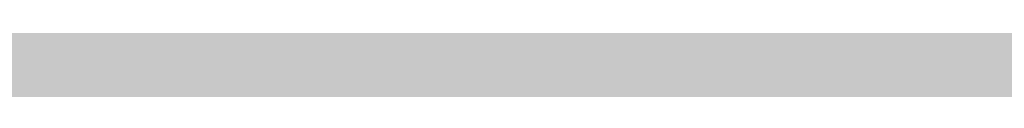
# Model space of a CAD drawing. Units: feet. Extents: x 3168 to 4724, y 827 to 1477.
# Tile 133 of 256: x 3300.8583 to 3301.1298, y 1099.0007 to 1099.0148. Entities that reach past the tile are written whole.
import ezdxf

# ---------------------------------------------------------------- set-up
doc = ezdxf.new("R2010")
doc.units = ezdxf.units.FT
doc.layers.add('A-ELEV', color=7, linetype='Continuous', lineweight=35)
doc.layers.add('A-ELEV-PATT', color=8, linetype='Continuous', lineweight=13)

msp = doc.modelspace()

# ---------------------------------------------------------------- hatches: boundary and pattern name
at = {"layer": 'A-ELEV-PATT'}
h = msp.add_hatch(color=256, dxfattribs=at)
h.dxf.hatch_style = 1
edge = h.paths.add_edge_path()
edge.add_ellipse((3552.90576, 979.22014), major_axis=(36.74492, 0), ratio=0.48484848, start_angle=0, end_angle=360)
edge = h.paths.add_edge_path()
edge.add_ellipse((3559.89164, 929.25228), major_axis=(36.74492, 0), ratio=0.48484848, start_angle=0, end_angle=360)
edge = h.paths.add_edge_path()
edge.add_line((3299.31681, 1198.60608), (3479.91671, 1198.60608))
edge.add_line((3479.91671, 1198.60608), (3479.91671, 1209.86857))
edge.add_spline(control_points=[(3479.91671, 1209.86857), (3464.30116, 1209.86857), (3448.6856, 1209.86857), (3410.94914, 1209.86857), (3388.82823, 1209.86857), (3355.64688, 1209.86857), (3344.58642, 1209.86857), (3327.99574, 1209.86857), (3322.46552, 1209.86857), (3314.17018, 1209.86857), (3311.40507, 1209.86857), (3307.2574, 1209.86857), (3305.87484, 1209.86857), (3303.801, 1209.86857), (3303.10973, 1209.86857), (3302.07281, 1209.86857), (3301.72717, 1209.86857), (3301.20871, 1209.86857), (3301.03589, 1209.86857), (3300.77666, 1209.86857), (3300.69025, 1209.86857), (3300.56064, 1209.86857), (3300.51743, 1209.86857), (3300.45263, 1209.86857), (3300.43102, 1209.86857), (3300.39862, 1209.86857), (3300.38782, 1209.86857), (3300.36622, 1209.86857), (3300.34568, 1209.86857), (3300.34555, 1209.86857), (3300.3455, 1209.86857), (3300.3433, 1209.86857), (3300.34115, 1209.86857), (3300.33791, 1209.86857), (3300.33683, 1209.86857), (3300.33394, 1209.86857), (3300.33213, 1209.86857), (3300.32552, 1209.86858), (3300.32071, 1209.86858), (3300.31092, 1209.86859), (3300.30595, 1209.8686), (3300.29051, 1209.86862), (3300.28005, 1209.86865), (3300.23243, 1209.86878), (3300.1953, 1209.86895), (3299.95107, 1209.87061), (3299.74482, 1209.87433), (3299.43683, 1209.88326), (3299.33439, 1209.88679), (3299.18108, 1209.89292), (3299.13003, 1209.8951), (3298.65222, 1209.9168), (3298.22946, 1209.94572), (3297.60163, 1210.00237), (3297.3934, 1210.02346), (3297.08265, 1210.05831), (3296.97933, 1210.07046), (3296.29295, 1210.15486), (3295.71815, 1210.24336), (3294.86872, 1210.39885), (3294.5877, 1210.45448), (3294.16934, 1210.54335), (3294.03042, 1210.57388), (3291.70715, 1211.1012), (3289.65359, 1211.81344), (3285.77626, 1213.56399), (3283.95141, 1214.60348), (3280.51216, 1216.98008), (3278.89724, 1218.31759), (3276.37991, 1220.82949), (3275.41604, 1221.91774), (3274.03934, 1223.7077), (3273.58104, 1224.34953), (3273.14323, 1225.01632)], knot_values=[39.119033, 39.119033, 39.119033, 39.119033, 39.286353, 39.286353, 39.523379, 39.523379, 39.641892, 39.641892, 39.701148, 39.701148, 39.730777, 39.730777, 39.745591, 39.745591, 39.752998, 39.752998, 39.756701, 39.756701, 39.758553, 39.758553, 39.759479, 39.759479, 39.759942, 39.759942, 39.760173, 39.760173, 39.760289, 39.760289, 39.760405, 39.760405, 39.760463, 39.760463, 39.763389, 39.763389, 39.764851, 39.764851, 39.767304, 39.767304, 39.773825, 39.773825, 39.78057, 39.78057, 39.79477, 39.79477, 39.845194, 39.845194, 40.126715, 40.126715, 40.267476, 40.267476, 40.337856, 40.337856, 40.927023, 40.927023, 41.221606, 41.221606, 41.368898, 41.368898, 42.202622, 42.202622, 42.619485, 42.619485, 42.827916, 42.827916, 46.118323, 46.118323, 49.408731, 49.408731, 52.699139, 52.699139, 54.927489, 54.927489, 56.104228, 56.104228, 56.104228, 56.104228], weights=[1, 1, 1, 1, 1, 1, 1, 1, 1, 1, 1, 1, 1, 1, 1, 1, 1, 1, 1, 1, 1, 1, 1, 1, 1, 1, 1, 1, 1, 1, 1, 1, 1, 1, 1, 1, 1, 1, 1, 1, 1, 1, 1, 1, 1, 1, 1, 1, 1, 1, 1, 1, 1, 1, 1, 1, 1, 1, 1, 1, 1, 1, 1, 1, 1, 1, 1, 1, 1, 1, 1, 1, 1, 1], degree=3, periodic=0)
edge.add_line((3273.14323, 1225.01632), (3273.14323, 1099.01632))
edge.add_line((3273.14323, 1099.01632), (3299.31681, 1099.01632))
edge.add_line((3299.31681, 1099.01632), (3299.31681, 1198.60608))
edge = h.paths.add_edge_path()
edge.add_line((3304.75844, 1324.15806), (3479.91671, 1324.15806))
edge.add_line((3479.91671, 1324.15806), (3479.91671, 1335.71462))
edge.add_line((3479.91671, 1335.71462), (3269.16163, 1335.71462))
edge.add_spline(control_points=[(3269.16163, 1335.71462), (3264.02423, 1335.71462), (3258.36412, 1328.95819), (3259.26431, 1323.90027)], knot_values=[0, 0, 0, 0, 15.412191, 15.412191, 15.412191, 15.412191], degree=3, periodic=0)
edge.add_line((3259.26431, 1323.90027), (3265.51685, 1288.76913))
edge.add_line((3265.51685, 1288.76913), (3275.2651, 1261.54563))
edge.add_line((3275.2651, 1261.54563), (3304.75844, 1261.54563))
edge.add_line((3304.75844, 1261.54563), (3304.75844, 1324.15806))
h = msp.add_hatch(color=256, dxfattribs=at)
h.dxf.hatch_style = 1
h.paths.add_polyline_path([(3384.52525, 1099.01632), (3335.02917, 1099.01632), (3299.31681, 1099.01632), (3273.14323, 1099.01632), (3217.56536, 1099.01632), (3168.06928, 827.11626), (3335.02917, 827.11626)])

# ---------------------------------------------------------------- linework, layer by layer
at = {"layer": 'A-ELEV'}
msp.add_open_spline([(3808.5202, 1099.01632), (3808.5202, 1141.41324), (3808.5202, 1183.81015), (3808.5202, 1226.63532), (3808.5202, 1227.06358), (3808.5202, 1227.49183), (3811.49187, 1248.99467), (3814.46354, 1270.49752), (3817.46523, 1292.21756), (3817.49525, 1292.43476), (3817.52526, 1292.65196), (3817.5728, 1310.10675), (3817.62034, 1327.56153), (3817.66788, 1345.01632), (3817.66788, 1345.45796), (3817.66788, 1345.89961), (3817.66788, 1346.45605), (3817.66788, 1346.57084), (3817.66788, 1346.75289), (3817.66788, 1346.82014), (3817.66788, 1346.93487), (3817.66788, 1346.98234), (3817.66788, 1347.03859), (3817.66788, 1347.04736), (3817.66788, 1347.07366), (3817.66788, 1347.0593), (3817.66788, 1347.06155), (3817.66788, 1347.06267), (3817.66788, 1347.06603), (3817.66787, 1347.06827), (3817.66787, 1347.075), (3817.66787, 1347.07949), (3817.66785, 1347.09294), (3817.66783, 1347.1019), (3817.66777, 1347.12879), (3817.6677, 1347.1467), (3817.66743, 1347.20042), (3817.66716, 1347.23619), (3817.6661, 1347.34338), (3817.66504, 1347.41469), (3817.66081, 1347.62809), (3817.65661, 1347.76971), (3817.63997, 1348.19249), (3817.62351, 1348.47159), (3817.55909, 1349.30007), (3817.49612, 1349.84059), (3817.25543, 1351.42416), (3817.02632, 1352.42879), (3816.30687, 1354.88891), (3815.74375, 1356.26873), (3814.46396, 1358.81921), (3813.74641, 1359.99097), (3812.19584, 1362.17234), (3811.36225, 1363.18212), (3809.58884, 1365.06901), (3808.64882, 1365.94611), (3806.65426, 1367.57962), (3805.5997, 1368.33615), (3803.35289, 1369.72233), (3802.16054, 1370.35239), (3799.60081, 1371.45359), (3798.23269, 1371.92548), (3795.28008, 1372.63462), (3793.69315, 1372.87207), (3791.86944, 1372.92648), (3791.74086, 1372.92922), (3791.35337, 1372.9341), (3791.09271, 1372.9329), (3790.30412, 1372.91507), (3789.76954, 1372.88419), (3789.20919, 1372.83024), (3789.19062, 1372.82842), (3789.13489, 1372.82291), (3789.0977, 1372.81914), (3789.04844, 1372.81401), (3789.0364, 1372.81274), (3789.00026, 1372.80892), (3788.97615, 1372.80633), (3788.9494, 1372.8034), (3788.94679, 1372.80312), (3788.94257, 1372.80266), (3788.94097, 1372.80248), (3788.93857, 1372.80222), (3788.93778, 1372.80213), (3788.93539, 1372.80187), (3788.86753, 1372.7944), (3788.75687, 1372.78223), (3788.70153, 1372.77614), (3788.53553, 1372.75788), (3788.42486, 1372.74571), (3788.09286, 1372.70918), (3787.87152, 1372.68484), (3787.20751, 1372.61179), (3786.76483, 1372.5631), (3785.43681, 1372.41701), (3784.55147, 1372.31962), (3781.89542, 1372.02744), (3780.12473, 1371.83266), (3774.81265, 1371.24831), (3771.27126, 1370.85874), (3760.64709, 1369.69004), (3753.56431, 1368.9109), (3732.31597, 1366.5735), (3718.15042, 1365.01523), (3694.00676, 1362.35933), (3684.02866, 1361.26169), (3674.05056, 1360.16406), (3664.60066, 1360.16406), (3655.15077, 1360.16406), (3626.80108, 1360.16406), (3607.90129, 1360.16406), (3551.20192, 1360.16406), (3513.40234, 1360.16406), (3467.72518, 1360.16406), (3459.8476, 1360.16406), (3436.21487, 1360.16406), (3420.45972, 1360.16406), (3373.19425, 1360.16406), (3341.68395, 1360.16406), (3302.84816, 1360.16406), (3295.52269, 1360.16406), (3286.03829, 1360.16406), (3283.87937, 1360.16406), (3277.40261, 1360.16406), (3273.08477, 1360.16406), (3267.73285, 1360.16406), (3266.69877, 1360.16406), (3263.59652, 1360.16406), (3261.52835, 1360.16406), (3259.23694, 1360.16406), (3259.0137, 1360.16406), (3258.34396, 1360.16406), (3257.89747, 1360.16406), (3257.431, 1360.16406), (3257.41102, 1360.16406), (3257.37057, 1360.16406), (3257.37547, 1360.16406), (3257.3746, 1360.16406), (3257.37394, 1360.16406), (3257.37196, 1360.16406), (3257.37064, 1360.16406), (3257.36667, 1360.16406), (3257.36403, 1360.16406), (3257.35611, 1360.16405), (3257.35083, 1360.16405), (3257.33499, 1360.16402), (3257.32443, 1360.164), (3257.29277, 1360.1639), (3257.27168, 1360.1638), (3257.20844, 1360.1634), (3257.16634, 1360.163), (3257.04021, 1360.16139), (3256.95635, 1360.15978), (3256.7055, 1360.15339), (3256.53924, 1360.14704), (3256.04357, 1360.12192), (3255.7173, 1360.0971), (3254.75245, 1360.00048), (3254.12797, 1359.90651), (3252.18007, 1359.52533), (3250.94157, 1359.14399), (3248.67018, 1358.24329), (3247.63574, 1357.72383), (3245.73263, 1356.60347), (3244.86339, 1356.00206), (3243.25311, 1354.74287), (3242.51197, 1354.08473), (3240.75105, 1352.34478), (3239.80096, 1351.22957), (3238.08777, 1348.87244), (3237.32469, 1347.63036), (3235.98251, 1344.97163), (3235.40221, 1343.55491), (3234.59108, 1340.81546), (3234.31088, 1339.54355), (3233.97649, 1336.80256), (3233.92211, 1335.33088), (3234.14892, 1332.59127), (3234.34953, 1331.3672), (3234.71989, 1329.99937), (3234.75242, 1329.88336), (3234.85362, 1329.5348), (3234.92589, 1329.30168), (3235.02484, 1329.00255), (3235.04692, 1328.93693), (3235.07764, 1328.84724), (3235.08592, 1328.8232), (3235.11094, 1328.75106), (3235.12783, 1328.70296), (3235.14799, 1328.64624), (3235.15106, 1328.63763), (3235.1561, 1328.62353), (3235.15806, 1328.61803), (3235.16021, 1328.61203), (3235.16561, 1328.59694), (3235.1801, 1328.55649), (3235.19026, 1328.5281), (3235.22076, 1328.44295), (3235.24108, 1328.38618), (3235.30207, 1328.21587), (3235.34273, 1328.10232), (3235.4647, 1327.7617), (3235.54601, 1327.53462), (3235.78995, 1326.85338), (3235.95258, 1326.39922), (3236.44046, 1325.03674), (3236.76571, 1324.12841), (3237.74148, 1321.40345), (3238.39198, 1319.5868), (3240.34351, 1314.13687), (3241.64452, 1310.50358), (3245.54757, 1299.60371), (3248.14961, 1292.33713), (3255.95571, 1270.53739), (3261.15977, 1256.00423), (3267.38762, 1238.612), (3268.4114, 1235.75294), (3269.51038, 1232.68386), (3269.58558, 1232.47385), (3269.70661, 1232.13585), (3269.75244, 1232.00786), (3269.82733, 1231.79873), (3269.85638, 1231.7176), (3269.90632, 1231.57812), (3269.92721, 1231.51978), (3269.97247, 1231.39341), (3269.99683, 1231.32537), (3270.0265, 1231.24251), (3270.03181, 1231.22768), (3270.04028, 1231.20402), (3270.03922, 1231.20698), (3270.03936, 1231.2066), (3270.03943, 1231.20641), (3270.03963, 1231.20585), (3270.03977, 1231.20547), (3270.04017, 1231.20433), (3270.04044, 1231.20358), (3270.04125, 1231.20131), (3270.0418, 1231.1998), (3270.04342, 1231.19527), (3270.0445, 1231.19225), (3270.04776, 1231.18318), (3270.04993, 1231.17714), (3270.05644, 1231.15903), (3270.06079, 1231.14696), (3270.07387, 1231.11076), (3270.08261, 1231.08666), (3270.10894, 1231.01441), (3270.1266, 1230.96635), (3270.17993, 1230.82246), (3270.21595, 1230.72692), (3270.32532, 1230.44151), (3270.40003, 1230.25281), (3270.62925, 1229.69144), (3270.78888, 1229.3235), (3271.28649, 1228.23832), (3271.6431, 1227.53975), (3272.77586, 1225.51528), (3273.61417, 1224.2605), (3275.41604, 1221.91774), (3276.37991, 1220.82949), (3278.89724, 1218.31759), (3280.51216, 1216.98008), (3283.95141, 1214.60348), (3285.77626, 1213.56399), (3289.65359, 1211.81344), (3291.70715, 1211.1012), (3294.03042, 1210.57388), (3294.16934, 1210.54335), (3294.5877, 1210.45448), (3294.86872, 1210.39885), (3295.71815, 1210.24336), (3296.29295, 1210.15486), (3296.97933, 1210.07046), (3297.08265, 1210.05831), (3297.3934, 1210.02346), (3297.60163, 1210.00237), (3298.22946, 1209.94572), (3298.65222, 1209.9168), (3299.13003, 1209.8951), (3299.18108, 1209.89292), (3299.33439, 1209.88679), (3299.43683, 1209.88326), (3299.74482, 1209.87433), (3299.95107, 1209.87061), (3300.1953, 1209.86895), (3300.23243, 1209.86878), (3300.28005, 1209.86865), (3300.29051, 1209.86862), (3300.30595, 1209.8686), (3300.31092, 1209.86859), (3300.32071, 1209.86858), (3300.32552, 1209.86858), (3300.33213, 1209.86857), (3300.33394, 1209.86857), (3300.33683, 1209.86857), (3300.33791, 1209.86857), (3300.34115, 1209.86857), (3300.3433, 1209.86857), (3300.3455, 1209.86857), (3300.34555, 1209.86857), (3300.34568, 1209.86857), (3300.36622, 1209.86857), (3300.38782, 1209.86857), (3300.39862, 1209.86857), (3300.43102, 1209.86857), (3300.45263, 1209.86857), (3300.51743, 1209.86857), (3300.56064, 1209.86857), (3300.69025, 1209.86857), (3300.77666, 1209.86857), (3301.03589, 1209.86857), (3301.20871, 1209.86857), (3301.72717, 1209.86857), (3302.07281, 1209.86857), (3303.10973, 1209.86857), (3303.801, 1209.86857), (3305.87484, 1209.86857), (3307.2574, 1209.86857), (3311.40507, 1209.86857), (3314.17018, 1209.86857), (3322.46552, 1209.86857), (3327.99574, 1209.86857), (3344.58642, 1209.86857), (3355.64688, 1209.86857), (3388.82823, 1209.86857), (3410.94914, 1209.86857), (3477.31185, 1209.86857), (3521.55366, 1209.86857), (3566.83618, 1209.86857), (3567.87689, 1209.86857), (3570.99902, 1209.86857), (3573.08043, 1209.86857), (3575.7814, 1209.86857), (3576.40094, 1209.86857), (3577.29582, 1209.86857), (3577.57115, 1209.86857), (3578.39715, 1209.86857), (3578.94781, 1209.86857), (3579.75649, 1209.86857), (3580.01451, 1209.86857), (3580.34274, 1209.86857), (3580.32686, 1209.86857), (3580.32717, 1209.86857), (3580.32732, 1209.86857), (3580.32778, 1209.86857), (3580.32809, 1209.86857), (3580.329, 1209.86857), (3580.32961, 1209.86857), (3580.33145, 1209.86857), (3580.33267, 1209.86857), (3580.33633, 1209.86857), (3580.33878, 1209.86857), (3580.34611, 1209.86856), (3580.35099, 1209.86856), (3580.36566, 1209.86854), (3580.37544, 1209.86852), (3580.4048, 1209.86845), (3580.42439, 1209.86838), (3580.48318, 1209.86808), (3580.52244, 1209.86779), (3580.64036, 1209.86662), (3580.71919, 1209.86545), (3580.95632, 1209.86077), (3581.11522, 1209.85607), (3581.59416, 1209.83723), (3581.91642, 1209.81833), (3582.88995, 1209.74243), (3583.54799, 1209.66617), (3585.53183, 1209.36062), (3586.86722, 1209.05389), (3589.47155, 1208.25247), (3590.74024, 1207.75785), (3591.99545, 1207.1588), (3592.05781, 1207.12874), (3592.24424, 1207.03795), (3592.36768, 1206.97663), (3592.73528, 1206.79036), (3592.97675, 1206.6631), (3593.24454, 1206.51644), (3593.27473, 1206.49982), (3593.36512, 1206.44984), (3593.42511, 1206.41633), (3593.60431, 1206.31529), (3593.72273, 1206.24721), (3593.85721, 1206.1684), (3593.87436, 1206.15832), (3593.92574, 1206.12804), (3593.9599, 1206.1078), (3594.06209, 1206.0469), (3594.12983, 1206.00607), (3594.20844, 1205.95817), (3594.21968, 1205.9513), (3594.25339, 1205.93069), (3594.27582, 1205.91692), (3594.34297, 1205.87554), (3594.38756, 1205.84785), (3594.43362, 1205.81905), (3594.43526, 1205.81802), (3594.44017, 1205.81495), (3594.44345, 1205.81289), (3594.44712, 1205.81059), (3594.44752, 1205.81035), (3594.44869, 1205.80961), (3594.44948, 1205.80912), (3594.45037, 1205.80856), (3594.45047, 1205.8085), (3594.4506, 1205.80842), (3594.4674, 1205.79789), (3594.49327, 1205.78167), (3594.5062, 1205.77357), (3594.54501, 1205.74925), (3594.57088, 1205.73303), (3594.64849, 1205.6844), (3594.70023, 1205.65197), (3594.85544, 1205.55469), (3594.95892, 1205.48984), (3595.26936, 1205.29528), (3595.47631, 1205.16558), (3596.09719, 1204.77646), (3596.5111, 1204.51705), (3597.75284, 1203.73883), (3598.58067, 1203.22001), (3601.06415, 1201.66355), (3602.71981, 1200.62591), (3607.68677, 1197.513), (3610.99809, 1195.43773), (3620.93202, 1189.2119), (3627.55464, 1185.06135), (3647.42251, 1172.60971), (3660.66775, 1164.30861), (3700.40348, 1139.40531), (3726.89397, 1122.80312), (3757.20572, 1103.80605), (3761.02697, 1101.41118), (3764.84822, 1099.01632), (3745.32827, 1099.01632), (3725.80832, 1099.01632), (3706.28837, 1099.01632), (3706.28837, 1108.45324), (3706.28837, 1117.89016), (3706.28837, 1127.32708), (3710.75075, 1127.32708), (3715.21314, 1127.32708), (3719.67553, 1127.32708)], degree=3, knots=[0, 0, 0, 0, 0.982037, 0.982037, 0.991957, 0.991957, 0.991957, 1.966522, 1.966522, 1.976367, 1.976367, 1.976367, 2.976367, 2.976367, 2.976367, 3.00169, 3.00169, 3.008272, 3.008272, 3.012129, 3.012129, 3.014851, 3.014851, 3.015353, 3.015353, 3.016359, 3.016359, 3.017365, 3.017365, 3.019376, 3.019376, 3.023398, 3.023398, 3.031442, 3.031442, 3.047531, 3.047531, 3.079708, 3.079708, 3.144063, 3.144063, 3.272772, 3.272772, 3.53019, 3.53019, 4.045026, 4.045026, 5.074698, 5.074698, 6.700878, 6.700878, 8.327058, 8.327058, 9.953238, 9.953238, 11.579418, 11.579418, 13.205598, 13.205598, 14.831778, 14.831778, 16.457958, 16.457958, 18.084138, 18.084138, 18.206872, 18.206872, 18.45234, 18.45234, 18.943275, 18.943275, 18.960093, 18.960093, 18.993729, 18.993729, 19.00461, 19.00461, 19.026374, 19.026374, 19.028737, 19.028737, 19.03018, 19.03018, 19.030897, 19.030897, 19.032332, 19.032332, 19.033766, 19.033766, 19.036636, 19.036636, 19.042374, 19.042374, 19.053851, 19.053851, 19.076805, 19.076805, 19.122714, 19.122714, 19.21453, 19.21453, 19.398163, 19.398163, 19.765429, 19.765429, 20.024128, 20.024128, 20.024128, 20.092031, 20.092031, 20.227836, 20.227836, 20.499446, 20.499446, 20.556051, 20.556051, 20.66926, 20.66926, 20.895678, 20.895678, 20.948316, 20.948316, 20.963829, 20.963829, 20.994855, 20.994855, 21.002285, 21.002285, 21.017146, 21.017146, 21.01875, 21.01875, 21.021959, 21.021959, 21.022102, 21.022102, 21.022249, 21.022249, 21.022708, 21.022708, 21.023627, 21.023627, 21.025464, 21.025464, 21.029138, 21.029138, 21.036486, 21.036486, 21.051183, 21.051183, 21.080575, 21.080575, 21.139361, 21.139361, 21.256932, 21.256932, 21.492073, 21.492073, 21.962356, 21.962356, 23.01002, 23.01002, 24.057684, 24.057684, 25.105348, 25.105348, 26.153011, 26.153011, 27.776787, 27.776787, 29.400562, 29.400562, 31.024337, 31.024337, 32.278801, 32.278801, 33.533265, 33.533265, 34.467568, 34.467568, 34.553971, 34.553971, 34.726776, 34.726776, 34.775309, 34.775309, 34.793079, 34.793079, 34.82862, 34.82862, 34.834979, 34.834979, 34.839039, 34.839039, 34.839411, 34.839411, 34.840285, 34.840285, 34.842034, 34.842034, 34.845531, 34.845531, 34.852525, 34.852525, 34.866512, 34.866512, 34.894488, 34.894488, 34.950439, 34.950439, 35.062342, 35.062342, 35.286147, 35.286147, 35.733758, 35.733758, 35.821815, 35.821815, 35.828283, 35.828283, 35.832225, 35.832225, 35.834724, 35.834724, 35.836521, 35.836521, 35.838617, 35.838617, 35.839073, 35.839073, 35.839345, 35.839345, 35.839617, 35.839617, 35.840161, 35.840161, 35.841249, 35.841249, 35.843425, 35.843425, 35.847778, 35.847778, 35.856482, 35.856482, 35.873891, 35.873891, 35.908709, 35.908709, 35.978345, 35.978345, 36.117617, 36.117617, 36.396161, 36.396161, 36.953248, 36.953248, 38.067423, 38.067423, 40.295772, 40.295772, 42.524122, 42.524122, 45.81453, 45.81453, 49.104937, 49.104937, 52.395345, 52.395345, 52.603776, 52.603776, 53.020639, 53.020639, 53.854363, 53.854363, 54.001655, 54.001655, 54.296238, 54.296238, 54.885405, 54.885405, 54.955785, 54.955785, 55.096546, 55.096546, 55.378067, 55.378067, 55.42849, 55.42849, 55.442691, 55.442691, 55.449436, 55.449436, 55.455957, 55.455957, 55.458409, 55.458409, 55.459872, 55.459872, 55.462798, 55.462798, 55.462856, 55.462856, 55.462972, 55.462972, 55.463088, 55.463088, 55.463319, 55.463319, 55.463782, 55.463782, 55.464708, 55.464708, 55.46656, 55.46656, 55.470263, 55.470263, 55.47767, 55.47767, 55.492484, 55.492484, 55.522112, 55.522112, 55.581369, 55.581369, 55.699882, 55.699882, 55.936907, 55.936907, 56.410959, 56.410959, 56.42211, 56.42211, 56.444413, 56.444413, 56.451051, 56.451051, 56.454001, 56.454001, 56.459901, 56.459901, 56.462666, 56.462666, 56.463418, 56.463418, 56.464171, 56.464171, 56.465675, 56.465675, 56.468684, 56.468684, 56.474702, 56.474702, 56.486738, 56.486738, 56.51081, 56.51081, 56.558955, 56.558955, 56.655243, 56.655243, 56.847821, 56.847821, 57.232975, 57.232975, 58.003284, 58.003284, 59.543901, 59.543901, 62.625137, 62.625137, 68.787607, 68.787607, 74.950078, 74.950078, 75.27336, 75.27336, 75.919923, 75.919923, 77.213051, 77.213051, 77.377769, 77.377769, 77.707206, 77.707206, 78.366079, 78.366079, 78.462532, 78.462532, 78.655436, 78.655436, 79.041245, 79.041245, 79.105735, 79.105735, 79.234714, 79.234714, 79.492672, 79.492672, 79.502197, 79.502197, 79.521249, 79.521249, 79.523534, 79.523534, 79.528103, 79.528103, 79.528682, 79.528682, 79.528885, 79.528885, 79.529089, 79.529089, 79.529495, 79.529495, 79.530308, 79.530308, 79.531935, 79.531935, 79.535187, 79.535187, 79.541693, 79.541693, 79.554704, 79.554704, 79.580725, 79.580725, 79.632769, 79.632769, 79.736856, 79.736856, 79.94503, 79.94503, 80.361377, 80.361377, 80.421435, 80.421435, 80.421435, 81.421435, 81.421435, 81.421435, 82.421435, 82.421435, 82.421435, 83.421435, 83.421435, 83.421435, 83.421435], dxfattribs=at)

doc.saveas('drawing.dxf')
